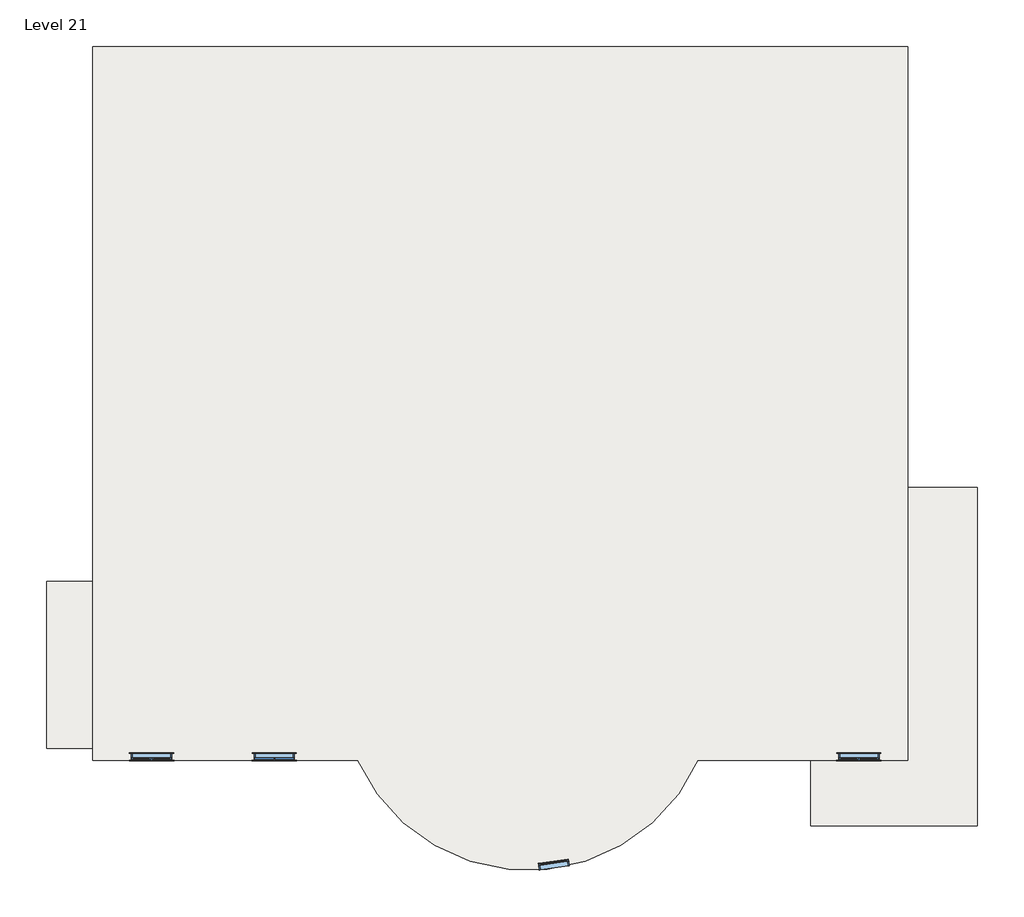
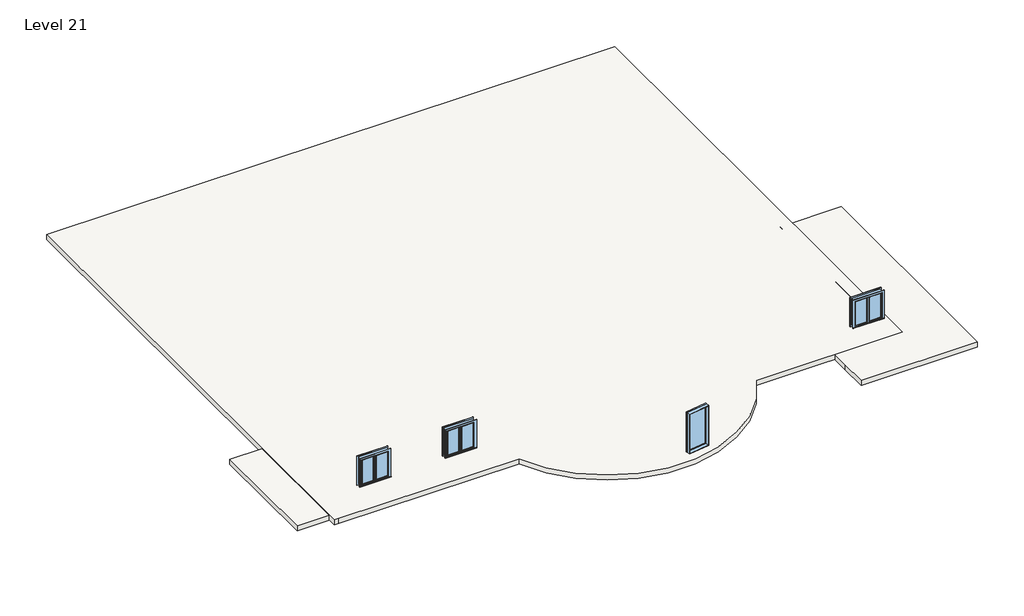
# One storey: 4 windows, 3 slabs.
"""IFC4 building model written with IfcOpenShell, lengths in millimetres."""

from ifc_helpers import new_model, si_unit, point, frame, frame_2d, origin, place, context, project, spatial, polyline, circle_curve, trimmed, segment, composite_curve, outline, extrude, transform, mapped, element, save
from components import window_0862ab64, window_9a779fa2

model = new_model("IFC4")

# Units and contexts
model_context = context("Model", 3, world=origin())
ifc_project = project(units=[si_unit("LENGTHUNIT", "METRE", prefix="MILLI")], contexts=[model_context])

# Site, building, storey
site = spatial("IfcSite", under=ifc_project)
building = spatial("IfcBuilding", under=site)
storey = spatial("IfcBuildingStorey", under=building, Name="Level 21", Elevation=32766.0)

# Slabs
placement = place(None, origin())
element("IfcSlab", 1, ObjectType="9\"", at=placement, inside=storey, context=model_context, shape_type="SweptSolid", body=[
    extrude(outline(composite_curve([segment(polyline([(-16607.9505427, 7461.1191779), (7979.2494573, 7461.1191779), (7979.2494573, -14078.0808221), (1652.8739931, -14078.0808221)]), True, "CONTINUOUS"), segment(trimmed(circle_curve(frame_2d((-3476.1505427, -11788.3650223)), 5616.9111737), [point((1652.8739931, -14078.0808221))], [point((-8605.1750786, -14078.0808221))], False, "CARTESIAN"), True, "CONTINUOUS"), segment(polyline([(-8605.1750786, -14078.0808221), (-16404.7505427, -14078.0808221), (-16607.9505427, -14078.0808221), (-16607.9505427, 7461.1191779)]), True, "CONTINUOUS")], self_intersect=False)), frame((0.0, 0.0, 32537.4), z_axis=(0.0, 0.0, 1.0), x_axis=(1.0, 0.0, 0.0)), (0.0, 0.0, 1.0), 228.6),
])
element("IfcSlab", 2, ObjectType="9\"", at=placement, inside=storey, context=model_context, shape_type="SweptSolid", body=[
    extrude(outline(polyline([(-17997.7050371, -8690.0239591), (-16626.1050371, -8690.0239591), (-16626.1050371, -13719.2239591), (-17997.7050371, -13719.2239591), (-17997.7050371, -8690.0239591)])), frame((0.0, 0.0, 32537.4), z_axis=(0.0, 0.0, 1.0), x_axis=(1.0, 0.0, 0.0)), (0.0, 0.0, 1.0), 228.6),
])
element("IfcSlab", 3, ObjectType="9\"", at=placement, inside=storey, context=model_context, shape_type="SweptSolid", body=[
    extrude(outline(polyline([(5053.8271821, -14840.0808221), (5053.8271821, -14078.0808221), (7238.2271821, -14078.0808221), (7441.4271821, -14078.0808221), (7441.4271821, -5848.4808221), (10083.0271821, -5848.4808221), (10083.0271821, -14840.0808221), (10083.0271821, -16059.2808221), (5053.8271821, -16059.2808221), (5053.8271821, -14840.0808221)])), frame((0.0, 0.0, 32537.4), z_axis=(0.0, 0.0, 1.0), x_axis=(1.0, 0.0, 0.0)), (0.0, 0.0, 1.0), 228.6),
])

# Windows
window_shape = window_0862ab64(model_context)
element("IfcWindow", 4, ObjectType="Casement Dbl with Trim : 48\" x 48\"", at=placement, inside=storey, context=model_context, shape_type="MappedRepresentation", body=[
    mapped(window_shape, transform((-14829.9505427, -13957.4308221, 32982.7338162), x_axis=(-1.0, 0.0, 0.0), y_axis=(0.0, -1.0, 0.0), z_axis=(0.0, 0.0, 1.0))),
])
element("IfcWindow", 5, ObjectType="Casement Dbl with Trim : 48\" x 48\"", at=placement, inside=storey, context=model_context, shape_type="MappedRepresentation", body=[
    mapped(window_shape, transform((-11129.6382271, -13957.4308221, 33012.8998834), x_axis=(-1.0, 0.0, 0.0), y_axis=(0.0, -1.0, 0.0), z_axis=(0.0, 0.0, 1.0))),
])
element("IfcWindow", 6, ObjectType="Casement Dbl with Trim : 48\" x 48\"", at=placement, inside=storey, context=model_context, shape_type="MappedRepresentation", body=[
    mapped(window_shape, transform((6506.0494573, -13957.4308221, 32766.0), x_axis=(-1.0, 0.0, 0.0), y_axis=(0.0, -1.0, 0.0), z_axis=(0.0, 0.0, 1.0))),
])
window_2_shape = window_9a779fa2(model_context)
element("IfcWindow", 7, ObjectType="Fixed : 36\" x 72\"", at=placement, inside=storey, context=model_context, shape_type="MappedRepresentation", body=[
    mapped(window_2_shape, transform((-2656.4484682, -17222.998006, 32766.0), x_axis=(0.9898258492754506, 0.1422841808007237, 0.0), y_axis=(-0.1422841808007237, 0.9898258492754506, 0.0), z_axis=(0.0, 0.0, 1.0))),
])

save(model, "model.ifc")

# Revit data of these elements
# Type "9\""
#   Assembly Code = "B1010"
#   Function = 0
#   Layers, outside or top first: 0' - 9" no material (function 1)
# Type "Casement Dbl with Trim : 48\" x 48\""
#   Type Mark = "10"
#   Construction Type Id = "GSP4R"
#   Assembly Code = "B2020100"
#   Analytic Construction = "1/8 in Pilkington single glazing"
#   Visual Light Transmittance = 0.9
#   Solar Heat Gain Coefficient = 0.78
#   Heat Transfer Coefficient (U) = 0.6496 BTU/(h·ft²·°F)
#   Height = 4' - 0"
#   Default Sill Height = 3' - 0"
#   Trim Projection - Ext. = 0' - 0 1/2"
#   Trim Projection - Int. = 0' - 0 3/4"
#   Trim Width - Exterior = 0' - 3 1/2"
#   Trim Width - Interior = 0' - 3 1/2"
#   Width = 4' - 0"
#   Window Inset = 0' - 0 3/4"
#   Define Thermal Properties by = 1
#   Glass Pane Material = Glass
#   Sash Material = Sash
#   Trim Exterior Material = Trim
#   Trim Interior Material = Trim
#   Wall Closure = (empty or 0)
# Type "Fixed : 36\" x 72\""
#   Type Mark = "9"
#   Construction Type Id = "GSP4R"
#   Assembly Code = "B2020100"
#   Analytic Construction = "1/8 in Pilkington single glazing"
#   Visual Light Transmittance = 0.9
#   Solar Heat Gain Coefficient = 0.78
#   Heat Transfer Coefficient (U) = 0.6496 BTU/(h·ft²·°F)
#   Height = 6' - 0"
#   Default Sill Height = 1' - 0"
#   Width = 3' - 0"
#   Window Inset = 0' - 0 3/4"
#   Define Thermal Properties by = 1
#   Glass Pane Material = Glass
#   Sash Material = Sash
#   Wall Closure = (empty or 0)
# Element 1 (IfcSlab, "9\"")
#   built-in parameter 1001955 = 1.5708 (stored number, unit not read)
#   Height Offset From Level = 0' - 0"
#   Phase Created = New Construction
#   Materials on its faces: "Default Floor"
# Element 2 (IfcSlab, "9\"")
#   built-in parameter 1001955 = 3.14159 (stored number, unit not read)
#   Height Offset From Level = 0' - 0"
#   Phase Created = New Construction
#   Materials on its faces: "Default Floor"
# Element 3 (IfcSlab, "9\"")
#   built-in parameter 1001955 = -1.5708 (stored number, unit not read)
#   Height Offset From Level = 0' - 0"
#   Phase Created = New Construction
#   Materials on its faces: "Default Floor"
# Element 4 (IfcWindow, "Casement Dbl with Trim : 48\" x 48\"")
#   Mark = "27"
#   Phase Created = New Construction
#   Materials on its faces: "Sash", "Trim", "Glass"
# Element 5 (IfcWindow, "Casement Dbl with Trim : 48\" x 48\"")
#   Mark = "28"
#   Phase Created = New Construction
#   Materials on its faces: "Sash", "Trim", "Glass"
# Element 6 (IfcWindow, "Casement Dbl with Trim : 48\" x 48\"")
#   Mark = "51"
#   Phase Created = New Construction
#   Materials on its faces: "Sash", "Trim", "Glass"
# Element 7 (IfcWindow, "Fixed : 36\" x 72\"")
#   Mark = "6"
#   Phase Created = New Construction
#   Materials on its faces: "Sash", "Glass"
# Materials
#   "Glass": class "Glass", colour RGB 0 128 192, transparency 0.75, Description = "Soda Lime Glass", Cost = 0
#   "Sash": class "Wood", colour RGB 224 178 126, transparency 0
#   "Trim": class "Wood", colour RGB 224 178 126, transparency 0
#   "Default Floor": colour RGB 128 128 128, transparency 0
